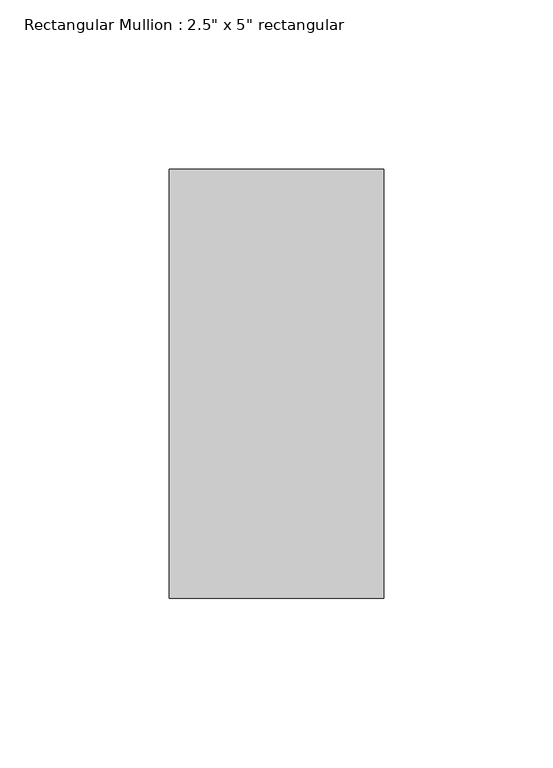
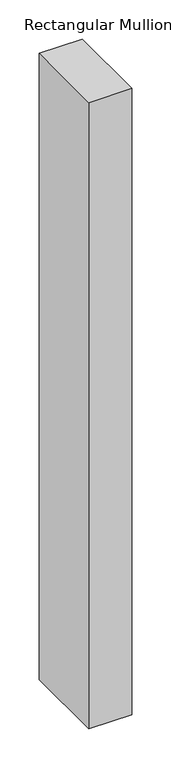
"""IFC4 building model written with IfcOpenShell, lengths in millimetres: member geometry."""

from ifc_helpers import new_model, si_unit, frame, origin, place, context, project, spatial, polyline, outline, extrude, source, transform, mapped, element, save


def member_801d2a92(model_context):
    return source(origin(), model_context, "Body", "SweptSolid", [
        extrude(outline(polyline([(0.0, 63.5), (0.0, -63.5), (-63.5, -63.5), (-63.5, 63.5), (0.0, 63.5)])), frame((0.0, 0.0, -977.634107), z_axis=(0.0, 0.0, 1.0), x_axis=(1.0, 0.0, 0.0)), (0.0, 0.0, 1.0), 977.634107),
    ])


if __name__ == "__main__":
    model = new_model("IFC4")
    model_context = context("Model", 3, world=origin())
    ifc_project = project(units=[si_unit("LENGTHUNIT", "METRE", prefix="MILLI")], contexts=[model_context])
    site = spatial("IfcSite", under=ifc_project)
    building = spatial("IfcBuilding", under=site)
    placement = place(None, origin())
    member_shape = member_801d2a92(model_context)
    element("IfcMember", 1, ObjectType="Rectangular Mullion : 2.5\" x 5\" rectangular", at=placement, inside=building, context=model_context, shape_type="MappedRepresentation", body=[
        mapped(member_shape, transform((0.0, 0.0, 0.0), x_axis=(1.0, 0.0, 0.0), y_axis=(0.0, 1.0, 0.0), z_axis=(0.0, 0.0, 1.0))),
    ])
    save(model, "model.ifc")

# Revit data of these elements
# Type "Rectangular Mullion : 2.5\" x 5\" rectangular"
#   built-in parameter 1007304 = 0.416667 (stored number, unit not read)
#   built-in parameter 1007301 = 0.104167 (stored number, unit not read)
#   built-in parameter 1007300 = 0.104167 (stored number, unit not read)
# Element 1 (IfcMember, "Rectangular Mullion : 2.5\" x 5\" rectangular")
#   Materials on its faces: "Roofing, EPDM Membrane"
# Materials
#   "Roofing, EPDM Membrane": class "Generic", colour RGB 127 127 127, transparency 0, Description = "EPDM roof membrane", Cost = 0
